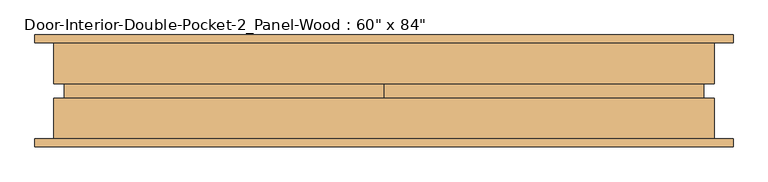
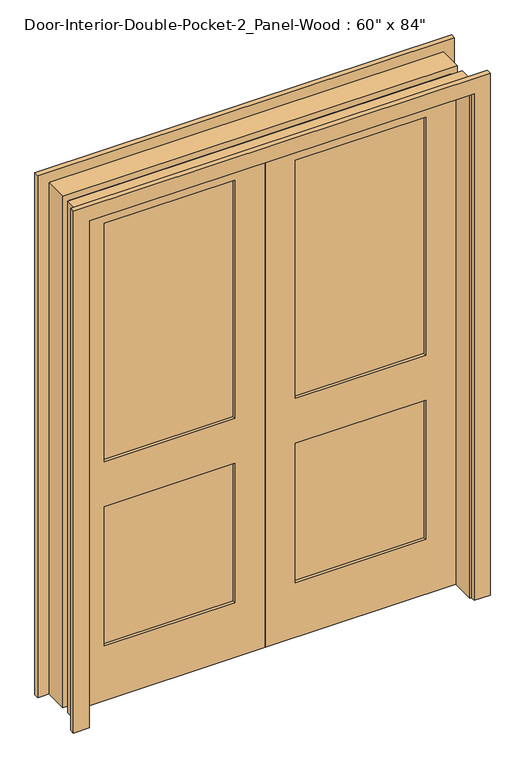
"""IFC4 building model written with IfcOpenShell, lengths in millimetres: door geometry."""

from ifc_helpers import new_model, si_unit, frame, origin, place, context, project, spatial, polyline, outline, extrude, source, transform, mapped, element, save


def door_7a66d0d1(model_context):
    return source(origin(), model_context, "Body", "SweptSolid", [
        extrude(outline(polyline([(0.0, 768.35), (0.0, 831.85), (2203.45, 831.85), (2203.45, -831.85), (0.0, -831.85), (0.0, -768.35), (2139.95, -768.35), (2139.95, 768.35), (0.0, 768.35)])), frame((0.0, 114.3, 0.0), z_axis=(0.0, 1.0, 0.0), x_axis=(0.0, 0.0, 1.0)), (0.0, 0.0, 1.0), 19.05),
        extrude(outline(polyline([(0.0, 768.35), (0.0, 831.85), (2203.45, 831.85), (2203.45, -831.85), (0.0, -831.85), (0.0, -768.35), (2139.95, -768.35), (2139.95, 768.35), (0.0, 768.35)])), frame((0.0, -133.35, 0.0), z_axis=(0.0, 1.0, 0.0), x_axis=(0.0, 0.0, 1.0)), (0.0, 0.0, 1.0), 19.05),
        extrude(outline(polyline([(2133.6, 0.0), (0.0, 0.0), (0.0, 762.0), (2133.6, 762.0), (2133.6, 0.0)]), holes=[polyline([(2014.5375, 120.65), (2014.5375, 641.35), (1009.65, 641.35), (1009.65, 120.65), (2014.5375, 120.65)]), polyline([(819.15, 120.65), (819.15, 641.35), (231.775, 641.35), (231.775, 120.65), (819.15, 120.65)])]), frame((0.0, -17.4625, 0.0), z_axis=(0.0, 1.0, 0.0), x_axis=(0.0, 0.0, 1.0)), (0.0, 0.0, 1.0), 34.925),
        extrude(outline(polyline([(641.35, -5.8208333), (120.65, -5.8208333), (120.65, 5.8208333), (641.35, 5.8208333), (641.35, -5.8208333)])), frame((0.0, 0.0, 1009.65), z_axis=(0.0, 0.0, 1.0), x_axis=(1.0, 0.0, 0.0)), (0.0, 0.0, 1.0), 1004.8875),
        extrude(outline(polyline([(641.35, -5.8208333), (120.65, -5.8208333), (120.65, 5.8208333), (641.35, 5.8208333), (641.35, -5.8208333)])), frame((0.0, 0.0, 231.775), z_axis=(0.0, 0.0, 1.0), x_axis=(1.0, 0.0, 0.0)), (0.0, 0.0, 1.0), 587.375),
        extrude(outline(polyline([(0.0, 787.4), (2159.0, 787.4), (2159.0, -787.4), (0.0, -787.4), (0.0, -762.0), (2133.6, -762.0), (2133.6, 762.0), (0.0, 762.0), (0.0, 787.4)])), frame((0.0, 17.4625, 0.0), z_axis=(0.0, 1.0, 0.0), x_axis=(0.0, 0.0, 1.0)), (0.0, 0.0, 1.0), 96.8375),
        extrude(outline(polyline([(0.0, 787.4), (2159.0, 787.4), (2159.0, -787.4), (0.0, -787.4), (0.0, -762.0), (2133.6, -762.0), (2133.6, 762.0), (0.0, 762.0), (0.0, 787.4)])), frame((0.0, -114.3, 0.0), z_axis=(0.0, 1.0, 0.0), x_axis=(0.0, 0.0, 1.0)), (0.0, 0.0, 1.0), 96.8375),
        extrude(outline(polyline([(2133.6, -762.0), (0.0, -762.0), (0.0, 0.0), (2133.6, 0.0), (2133.6, -762.0)]), holes=[polyline([(2014.5375, -641.35), (2014.5375, -120.65), (1009.65, -120.65), (1009.65, -641.35), (2014.5375, -641.35)]), polyline([(819.15, -641.35), (819.15, -120.65), (231.775, -120.65), (231.775, -641.35), (819.15, -641.35)])]), frame((0.0, -17.4625, 0.0), z_axis=(0.0, 1.0, 0.0), x_axis=(0.0, 0.0, 1.0)), (0.0, 0.0, 1.0), 34.925),
        extrude(outline(polyline([(-120.65, -5.8208333), (-641.35, -5.8208333), (-641.35, 5.8208333), (-120.65, 5.8208333), (-120.65, -5.8208333)])), frame((0.0, 0.0, 1009.65), z_axis=(0.0, 0.0, 1.0), x_axis=(1.0, 0.0, 0.0)), (0.0, 0.0, 1.0), 1004.8875),
        extrude(outline(polyline([(-120.65, -5.8208333), (-641.35, -5.8208333), (-641.35, 5.8208333), (-120.65, 5.8208333), (-120.65, -5.8208333)])), frame((0.0, 0.0, 231.775), z_axis=(0.0, 0.0, 1.0), x_axis=(1.0, 0.0, 0.0)), (0.0, 0.0, 1.0), 587.375),
    ])


if __name__ == "__main__":
    model = new_model("IFC4")
    model_context = context("Model", 3, world=origin())
    ifc_project = project(units=[si_unit("LENGTHUNIT", "METRE", prefix="MILLI")], contexts=[model_context])
    site = spatial("IfcSite", under=ifc_project)
    building = spatial("IfcBuilding", under=site)
    placement = place(None, origin())
    door_shape = door_7a66d0d1(model_context)
    element("IfcDoor", 1, ObjectType="Door-Interior-Double-Pocket-2_Panel-Wood : 60\" x 84\"", at=placement, inside=building, context=model_context, shape_type="MappedRepresentation", body=[
        mapped(door_shape, transform((0.0, 0.0, 0.0), x_axis=(1.0, 0.0, 0.0), y_axis=(0.0, 1.0, 0.0), z_axis=(0.0, 0.0, 1.0))),
    ])
    save(model, "model.ifc")

# Revit data of these elements
# Type "Door-Interior-Double-Pocket-2_Panel-Wood : 60\" x 84\""
#   Type Mark = "9"
#   Assembly Code = "C1020300"
#   Analytic Construction = "Wooden"
#   Top Rail = 0' - 4 11/16"
#   Thickness = 0' - 1 3/8"
#   Thermal Resistance (R) = 2.5876 (h·ft²·°F)/BTU
#   Stiles = 0' - 4 3/4"
#   Rough Width = 10' - 2"
#   Rough Height = 7' - 4 1/2"
#   Panel Width = 2' - 6"
#   Lock Rail = 0' - 7 1/2"
#   Location [instance default] = 2' - 7"
#   Height = 7' - 0"
#   Width = 5' - 0"
#   Heat Transfer Coefficient (U) = 0.3865 BTU/(h·ft²·°F)
#   Bottom Rail = 0' - 9 1/8"
#   Panel Open [instance default] = no
#   Trim Material = Cherry
#   Panel Material = Cherry
#   Frame Material = Cherry
#   Visual Light Transmittance = 0
#   Solar Heat Gain Coefficient = 0
#   Wall Closure = (empty or 0)
#   Function = (empty or 0)
# Element 1 (IfcDoor, "Door-Interior-Double-Pocket-2_Panel-Wood : 60\" x 84\"")
#   Materials on its faces: "Cherry"
# Materials
#   "Cherry": class "Wood", colour RGB 226 177 128, transparency 0, Description = "Prunus Serotina", Cost = 0
